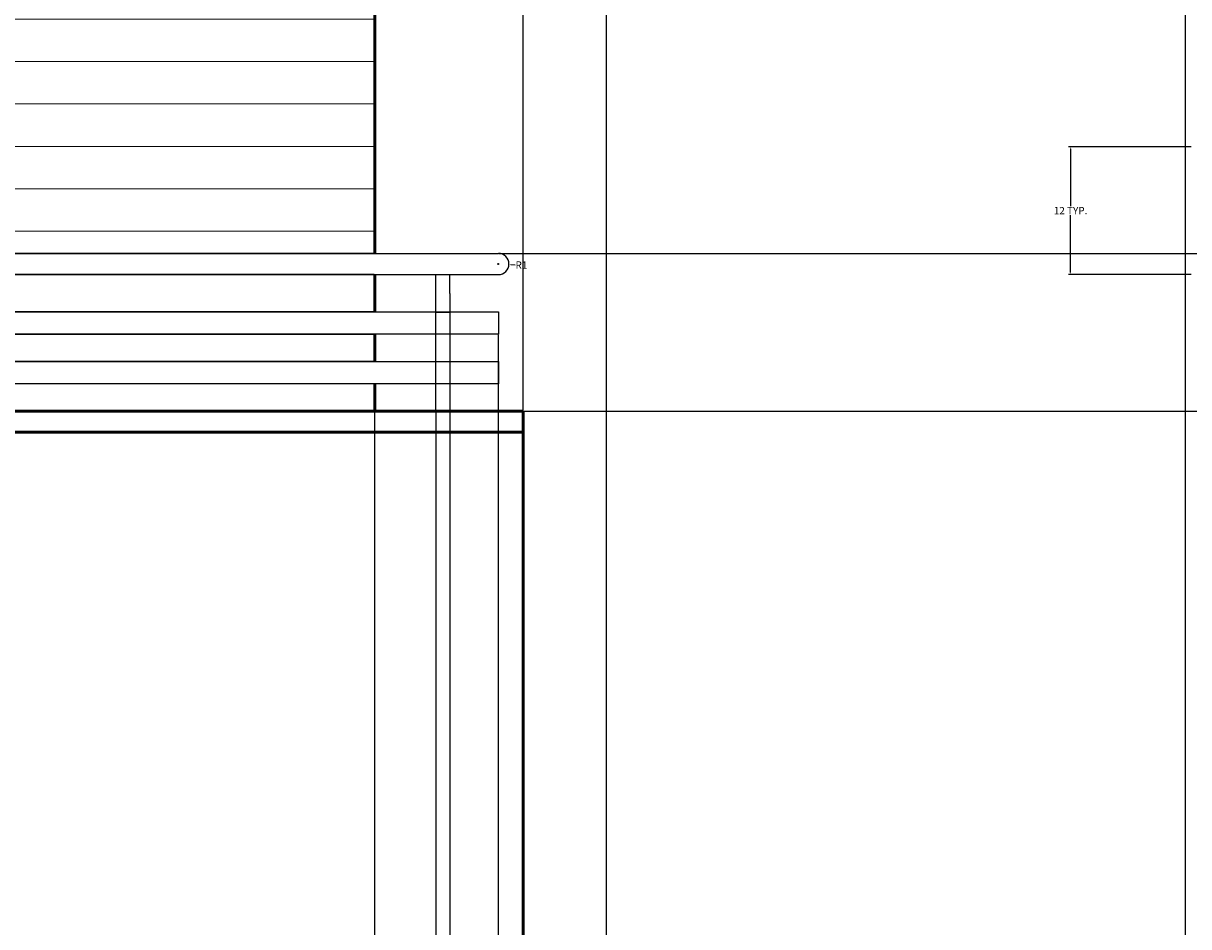
# Model space of a CAD drawing. Units: inches. Extents: x -139 to 346, y 72 to 413.
# Tile 9 of 18: x 66 to 175, y 242 to 328. Entities that reach past the tile are written whole.
import ezdxf

# ---------------------------------------------------------------- set-up
doc = ezdxf.new("R2010")
doc.units = ezdxf.units.IN
doc.header["$MEASUREMENT"] = 0
for name, color, linetype, lineweight in [('A-ANNO-DIMS', 2, 'Continuous', 18), ('A-ELEV-RAIL', 6, 'Continuous', 25), ('A-WALL', 7, 'Continuous', 50), ('A-WALL-PATT', 8, 'Continuous', 13)]:
    doc.layers.add(name, color=color, linetype=linetype, lineweight=lineweight)
doc.styles.get("Standard").update_dxf_attribs({"font": 'arial.ttf'})
doc.dimstyles.get("Standard").update_dxf_attribs({"dimtxt": 0.6875, "dimasz": 0.18, "dimexe": 0.18, "dimexo": 0.0625, "dimgap": 0.09, "dimtad": 0, "dimtih": 1, "dimtoh": 1, "dimdec": 4, "dimzin": 0, "dimdsep": 46, "dimlunit": 4, "dimtxsty": 'Standard', "dimcen": 0.09, "dimadec": 0, "dimazin": 0, "dimtfac": 1, "dimtdec": 4, "dimtofl": 0, "dimtmove": 0, "dimatfit": 3, "dimfxl": 1, "dimtolj": 1, "dimtzin": 0, "dimarcsym": 0})

# ---------------------------------------------------------------- blocks, each defined once
blk = doc.blocks.new('*D4')
at = {"layer": 'A-ANNO-DIMS', "color": 0, "lineweight": -2, "transparency": 16777216}
for p, q in [((175.61, 315.96), (164.06, 315.96)), ((164.24, 315.78), (164.24, 310.38)), ((164.24, 304.12), (164.24, 309.51)), ((175.61, 303.94), (164.06, 303.94))]:
    blk.add_line(p, q, dxfattribs=at)
at = {"layer": 'A-ANNO-DIMS', "color": 0, "transparency": 16777216}
for points in [[(164.21, 315.78), (164.27, 315.78), (164.24, 315.96)], [(164.21, 304.12), (164.27, 304.12), (164.24, 303.94)]]:
    blk.add_solid(points, dxfattribs=at)
at = {"layer": 'Defpoints', "color": 0, "transparency": 16777216}
for p in [(164.24, 315.96), (175.67, 315.96), (175.67, 303.94)]:
    blk.add_point(p, dxfattribs=at)
at = {"layer": 'A-ANNO-DIMS', "color": 0, "transparency": 16777216, "insert": (164.24, 309.95), "char_height": 0.6875, "attachment_point": 5}
blk.add_mtext('\\A1;12 TYP.', dxfattribs=at)
blk = doc.blocks.new('*D26')
at = {"layer": 'A-ANNO-DIMS', "color": 0, "lineweight": -2, "transparency": 16777216}
for p, q in [((98.67, 360.61), (98.67, 412.45)), ((98.85, 412.27), (104.18, 412.27)), ((112.47, 412.27), (107.15, 412.27)), ((112.65, 291.12), (112.65, 412.45))]:
    blk.add_line(p, q, dxfattribs=at)
at = {"layer": 'A-ANNO-DIMS', "color": 0, "transparency": 16777216}
for points in [[(98.85, 412.3), (98.85, 412.24), (98.67, 412.27)], [(112.47, 412.3), (112.47, 412.24), (112.65, 412.27)]]:
    blk.add_solid(points, dxfattribs=at)
at = {"layer": 'Defpoints', "color": 0, "transparency": 16777216}
for p in [(112.65, 412.27), (98.67, 360.54), (112.65, 291.06)]:
    blk.add_point(p, dxfattribs=at)
at = {"layer": 'A-ANNO-DIMS', "color": 0, "transparency": 16777216, "insert": (105.66, 412.27), "char_height": 0.688, "attachment_point": 5}
blk.add_mtext('\\A1;13.978', dxfattribs=at)
blk = doc.blocks.new('*D27')
at = {"layer": 'A-ANNO-DIMS', "color": 0, "lineweight": -2, "transparency": 16777216}
for p, q in [((112.65, 291.12), (112.65, 412.45)), ((112.83, 412.27), (142.91, 412.27)), ((175.49, 412.27), (145.41, 412.27)), ((175.67, 340.12), (175.67, 412.45))]:
    blk.add_line(p, q, dxfattribs=at)
at = {"layer": 'A-ANNO-DIMS', "color": 0, "transparency": 16777216}
for points in [[(112.83, 412.3), (112.83, 412.24), (112.65, 412.27)], [(175.49, 412.3), (175.49, 412.24), (175.67, 412.27)]]:
    blk.add_solid(points, dxfattribs=at)
at = {"layer": 'Defpoints', "color": 0, "transparency": 16777216}
for p in [(175.67, 412.27), (175.67, 340.05), (112.65, 291.06)]:
    blk.add_point(p, dxfattribs=at)
at = {"layer": 'A-ANNO-DIMS', "color": 0, "transparency": 16777216, "insert": (144.16, 412.27), "char_height": 0.688, "attachment_point": 5}
blk.add_mtext('\\A1;63.02', dxfattribs=at)
blk = doc.blocks.new('*D69')
at = {"layer": 'A-ANNO-DIMS', "color": 0, "lineweight": -2, "transparency": 16777216}
for p, q in [((120.51, 231.12), (120.51, 412.45)), ((120.69, 412.27), (146.54, 412.27)), ((174.89, 412.27), (149.04, 412.27)), ((175.07, 231.12), (175.07, 412.45))]:
    blk.add_line(p, q, dxfattribs=at)
at = {"layer": 'A-ANNO-DIMS', "color": 0, "transparency": 16777216}
for points in [[(120.69, 412.3), (120.69, 412.24), (120.51, 412.27)], [(174.89, 412.3), (174.89, 412.24), (175.07, 412.27)]]:
    blk.add_solid(points, dxfattribs=at)
at = {"layer": 'Defpoints', "color": 0, "transparency": 16777216}
for p in [(175.07, 412.27), (120.51, 231.06), (175.07, 231.06)]:
    blk.add_point(p, dxfattribs=at)
at = {"layer": 'A-ANNO-DIMS', "color": 0, "transparency": 16777216, "insert": (147.79, 412.27), "char_height": 0.688, "attachment_point": 5}
blk.add_mtext('\\A1;54.57', dxfattribs=at)
blk = doc.blocks.new('*D95')
at = {"layer": 'A-ANNO-DIMS', "color": 0, "lineweight": -2, "transparency": 16777216}
for p, q in [((98.61, 293.63), (-137.3, 293.63)), ((-137.12, 293.45), (-137.12, 292.78)), ((98.61, 291.06), (-137.3, 291.06)), ((-137.12, 291.24), (-137.12, 291.9))]:
    blk.add_line(p, q, dxfattribs=at)
at = {"layer": 'A-ANNO-DIMS', "color": 0, "transparency": 16777216}
for points in [[(-137.15, 293.45), (-137.09, 293.45), (-137.12, 293.63)], [(-137.15, 291.24), (-137.09, 291.24), (-137.12, 291.06)]]:
    blk.add_solid(points, dxfattribs=at)
at = {"layer": 'Defpoints', "color": 0, "transparency": 16777216}
for p in [(-137.12, 293.63), (98.67, 293.63), (98.67, 291.06)]:
    blk.add_point(p, dxfattribs=at)
at = {"layer": 'A-ANNO-DIMS', "color": 0, "transparency": 16777216, "insert": (-137.12, 292.34), "char_height": 0.688, "attachment_point": 5}
blk.add_mtext('\\A1;2.566', dxfattribs=at)
blk = doc.blocks.new('*D96')
at = {"layer": 'A-ANNO-DIMS', "color": 0, "lineweight": -2, "transparency": 16777216}
for p, q in [((98.61, 295.74), (-137.3, 295.74)), ((-137.12, 295.56), (-137.12, 295.12)), ((98.61, 293.63), (-137.3, 293.63)), ((-137.12, 293.81), (-137.12, 294.25))]:
    blk.add_line(p, q, dxfattribs=at)
at = {"layer": 'A-ANNO-DIMS', "color": 0, "transparency": 16777216}
for points in [[(-137.15, 295.56), (-137.09, 295.56), (-137.12, 295.74)], [(-137.15, 293.81), (-137.09, 293.81), (-137.12, 293.63)]]:
    blk.add_solid(points, dxfattribs=at)
at = {"layer": 'Defpoints', "color": 0, "transparency": 16777216}
for p in [(-137.12, 295.74), (98.67, 295.74), (98.67, 293.63)]:
    blk.add_point(p, dxfattribs=at)
at = {"layer": 'A-ANNO-DIMS', "color": 0, "transparency": 16777216, "insert": (-137.12, 294.68), "char_height": 0.688, "attachment_point": 5}
blk.add_mtext('\\A1;2.11', dxfattribs=at)
blk = doc.blocks.new('*D97')
at = {"layer": 'A-ANNO-DIMS', "color": 0, "lineweight": -2, "transparency": 16777216}
for p, q in [((98.61, 298.29), (-137.3, 298.29)), ((-137.12, 298.11), (-137.12, 297.46)), ((-137.12, 295.92), (-137.12, 296.57)), ((98.61, 295.74), (-137.3, 295.74))]:
    blk.add_line(p, q, dxfattribs=at)
at = {"layer": 'A-ANNO-DIMS', "color": 0, "transparency": 16777216}
for points in [[(-137.15, 298.11), (-137.09, 298.11), (-137.12, 298.29)], [(-137.15, 295.92), (-137.09, 295.92), (-137.12, 295.74)]]:
    blk.add_solid(points, dxfattribs=at)
at = {"layer": 'Defpoints', "color": 0, "transparency": 16777216}
for p in [(-137.12, 298.29), (98.67, 298.29), (98.67, 295.74)]:
    blk.add_point(p, dxfattribs=at)
at = {"layer": 'A-ANNO-DIMS', "color": 0, "transparency": 16777216, "insert": (-137.12, 297.02), "char_height": 0.688, "attachment_point": 5}
blk.add_mtext('\\A1;2.555', dxfattribs=at)
blk = doc.blocks.new('*D98')
at = {"layer": 'A-ANNO-DIMS', "color": 0, "lineweight": -2, "transparency": 16777216}
for p, q in [((98.61, 300.4), (-137.3, 300.4)), ((-137.12, 300.22), (-137.12, 299.78)), ((-137.12, 298.47), (-137.12, 298.91)), ((98.61, 298.29), (-137.3, 298.29))]:
    blk.add_line(p, q, dxfattribs=at)
at = {"layer": 'A-ANNO-DIMS', "color": 0, "transparency": 16777216}
for points in [[(-137.15, 300.22), (-137.09, 300.22), (-137.12, 300.4)], [(-137.15, 298.47), (-137.09, 298.47), (-137.12, 298.29)]]:
    blk.add_solid(points, dxfattribs=at)
at = {"layer": 'Defpoints', "color": 0, "transparency": 16777216}
for p in [(-137.12, 300.4), (98.67, 300.4), (98.67, 298.29)]:
    blk.add_point(p, dxfattribs=at)
at = {"layer": 'A-ANNO-DIMS', "color": 0, "transparency": 16777216, "insert": (-137.12, 299.35), "char_height": 0.688, "attachment_point": 5}
blk.add_mtext('\\A1;2.11', dxfattribs=at)
blk = doc.blocks.new('*D99')
at = {"layer": 'A-ANNO-DIMS', "color": 0, "lineweight": -2, "transparency": 16777216}
for p, q in [((98.61, 303.92), (-137.3, 303.92)), ((-137.12, 303.74), (-137.12, 302.6)), ((-137.12, 300.58), (-137.12, 301.72)), ((98.61, 300.4), (-137.3, 300.4))]:
    blk.add_line(p, q, dxfattribs=at)
at = {"layer": 'A-ANNO-DIMS', "color": 0, "transparency": 16777216}
for points in [[(-137.15, 303.74), (-137.09, 303.74), (-137.12, 303.92)], [(-137.15, 300.58), (-137.09, 300.58), (-137.12, 300.4)]]:
    blk.add_solid(points, dxfattribs=at)
at = {"layer": 'Defpoints', "color": 0, "transparency": 16777216}
for p in [(-137.12, 303.92), (98.67, 303.92), (98.67, 300.4)]:
    blk.add_point(p, dxfattribs=at)
at = {"layer": 'A-ANNO-DIMS', "color": 0, "transparency": 16777216, "insert": (-137.12, 302.16), "char_height": 0.688, "attachment_point": 5}
blk.add_mtext('\\A1;3.516', dxfattribs=at)
blk = doc.blocks.new('*D100')
at = {"layer": 'A-ANNO-DIMS', "color": 0, "lineweight": -2, "transparency": 16777216}
for p, q in [((98.61, 305.92), (-137.3, 305.92)), ((-137.12, 305.74), (-137.12, 305.36)), ((-137.12, 304.1), (-137.12, 304.49)), ((98.61, 303.92), (-137.3, 303.92))]:
    blk.add_line(p, q, dxfattribs=at)
at = {"layer": 'A-ANNO-DIMS', "color": 0, "transparency": 16777216}
for points in [[(-137.15, 305.74), (-137.09, 305.74), (-137.12, 305.92)], [(-137.15, 304.1), (-137.09, 304.1), (-137.12, 303.92)]]:
    blk.add_solid(points, dxfattribs=at)
at = {"layer": 'Defpoints', "color": 0, "transparency": 16777216}
for p in [(-137.12, 305.92), (98.67, 305.92), (98.67, 303.92)]:
    blk.add_point(p, dxfattribs=at)
at = {"layer": 'A-ANNO-DIMS', "color": 0, "transparency": 16777216, "insert": (-137.12, 304.92), "char_height": 0.688, "attachment_point": 5}
blk.add_mtext('\\A1;2', dxfattribs=at)
blk = doc.blocks.new('*D101')
at = {"layer": 'A-ANNO-DIMS', "color": 0, "lineweight": -2, "transparency": 16777216}
for p, q in [((110.39, 305.92), (344.39, 305.92)), ((344.21, 305.74), (344.21, 298.93)), ((344.21, 291.24), (344.21, 298.05)), ((112.71, 291.06), (344.39, 291.06))]:
    blk.add_line(p, q, dxfattribs=at)
at = {"layer": 'A-ANNO-DIMS', "color": 0, "transparency": 16777216}
for points in [[(344.18, 305.74), (344.24, 305.74), (344.21, 305.92)], [(344.18, 291.24), (344.24, 291.24), (344.21, 291.06)]]:
    blk.add_solid(points, dxfattribs=at)
at = {"layer": 'Defpoints', "color": 0, "transparency": 16777216}
for p in [(110.32, 305.92), (344.21, 305.92), (112.65, 291.06)]:
    blk.add_point(p, dxfattribs=at)
at = {"layer": 'A-ANNO-DIMS', "color": 0, "transparency": 16777216, "insert": (344.21, 298.49), "char_height": 0.688, "attachment_point": 5}
blk.add_mtext('\\A1;14.86', dxfattribs=at)
blk = doc.blocks.new('*D102')
at = {"layer": 'A-ANNO-DIMS', "color": 0, "lineweight": -2, "transparency": 16777216}
for p, q in [((98.67, 291), (98.67, 72.49)), ((104.42, 291), (104.42, 72.49)), ((98.85, 72.67), (100.3, 72.67)), ((104.24, 72.67), (102.79, 72.67))]:
    blk.add_line(p, q, dxfattribs=at)
at = {"layer": 'A-ANNO-DIMS', "color": 0, "transparency": 16777216}
for points in [[(98.85, 72.7), (98.85, 72.64), (98.67, 72.67)], [(104.24, 72.7), (104.24, 72.64), (104.42, 72.67)]]:
    blk.add_solid(points, dxfattribs=at)
at = {"layer": 'Defpoints', "color": 0, "transparency": 16777216}
for p in [(98.67, 291.06), (104.42, 291.06), (104.42, 72.67)]:
    blk.add_point(p, dxfattribs=at)
at = {"layer": 'A-ANNO-DIMS', "color": 0, "transparency": 16777216, "insert": (101.55, 72.67), "char_height": 0.688, "attachment_point": 5}
blk.add_mtext('\\A1;5.752', dxfattribs=at)
blk = doc.blocks.new('*D103')
at = {"layer": 'A-ANNO-DIMS', "color": 0, "lineweight": -2, "transparency": 16777216}
for p, q in [((104.42, 291), (104.42, 72.49)), ((105.74, 291), (105.74, 72.49)), ((104.6, 72.67), (105.56, 72.67)), ((105.74, 72.67), (105.92, 72.67))]:
    blk.add_line(p, q, dxfattribs=at)
at = {"layer": 'A-ANNO-DIMS', "color": 0, "transparency": 16777216}
for points in [[(104.6, 72.7), (104.6, 72.64), (104.42, 72.67)], [(105.56, 72.7), (105.56, 72.64), (105.74, 72.67)]]:
    blk.add_solid(points, dxfattribs=at)
at = {"layer": 'Defpoints', "color": 0, "transparency": 16777216}
for p in [(104.42, 291.06), (105.74, 291.06), (105.74, 72.67)]:
    blk.add_point(p, dxfattribs=at)
at = {"layer": 'A-ANNO-DIMS', "color": 0, "transparency": 16777216, "insert": (106.87, 72.67), "char_height": 0.688, "attachment_point": 5}
blk.add_mtext('\\A1;1.32', dxfattribs=at)
blk = doc.blocks.new('*D104')
at = {"layer": 'A-ANNO-DIMS', "color": 0, "lineweight": -2, "transparency": 16777216}
for p, q in [((110.32, 298.23), (110.32, 72.49)), ((105.74, 291), (105.74, 72.49)), ((105.92, 72.67), (106.77, 72.67)), ((110.14, 72.67), (109.29, 72.67))]:
    blk.add_line(p, q, dxfattribs=at)
at = {"layer": 'A-ANNO-DIMS', "color": 0, "transparency": 16777216}
for points in [[(105.92, 72.7), (105.92, 72.64), (105.74, 72.67)], [(110.14, 72.7), (110.14, 72.64), (110.32, 72.67)]]:
    blk.add_solid(points, dxfattribs=at)
at = {"layer": 'Defpoints', "color": 0, "transparency": 16777216}
for p in [(110.32, 298.29), (105.74, 291.06), (110.32, 72.67)]:
    blk.add_point(p, dxfattribs=at)
at = {"layer": 'A-ANNO-DIMS', "color": 0, "transparency": 16777216, "insert": (108.03, 72.67), "char_height": 0.688, "attachment_point": 5}
blk.add_mtext('\\A1;4.582', dxfattribs=at)
blk = doc.blocks.new('*D105')
at = {"layer": 'A-ANNO-DIMS', "color": 0, "lineweight": -2, "transparency": 16777216}
for p, q in [((110.32, 298.23), (110.32, 72.49)), ((112.65, 289), (112.65, 72.49)), ((110.5, 72.67), (112.47, 72.67)), ((112.65, 72.67), (112.83, 72.67))]:
    blk.add_line(p, q, dxfattribs=at)
at = {"layer": 'A-ANNO-DIMS', "color": 0, "transparency": 16777216}
for points in [[(110.5, 72.7), (110.5, 72.64), (110.32, 72.67)], [(112.47, 72.7), (112.47, 72.64), (112.65, 72.67)]]:
    blk.add_solid(points, dxfattribs=at)
at = {"layer": 'Defpoints', "color": 0, "transparency": 16777216}
for p in [(110.32, 298.29), (112.65, 289.06), (112.65, 72.67)]:
    blk.add_point(p, dxfattribs=at)
at = {"layer": 'A-ANNO-DIMS', "color": 0, "transparency": 16777216, "insert": (114.09, 72.67), "char_height": 0.688, "attachment_point": 5}
blk.add_mtext('\\A1;2.326', dxfattribs=at)
blk = doc.blocks.new('*D106')
at = {"layer": 'A-ANNO-DIMS', "color": 0, "lineweight": -2, "transparency": 16777216}
for p, q in [((110.23, 304.92), (110.41, 304.92)), ((110.32, 304.83), (110.32, 305.01)), ((111.92, 304.82), (111.5, 304.84))]:
    blk.add_line(p, q, dxfattribs=at)
at = {"layer": 'A-ANNO-DIMS', "color": 0, "transparency": 16777216}
blk.add_solid([(111.5, 304.87), (111.5, 304.81), (111.32, 304.86)], dxfattribs=at)
at = {"layer": 'Defpoints', "color": 0, "transparency": 16777216}
for p in [(110.32, 304.92), (111.32, 304.86)]:
    blk.add_point(p, dxfattribs=at)
at = {"layer": 'A-ANNO-DIMS', "color": 0, "transparency": 16777216, "insert": (112.5, 304.82), "char_height": 0.688, "attachment_point": 5}
blk.add_mtext('\\A1;R1', dxfattribs=at)

msp = doc.modelspace()

# ---------------------------------------------------------------- hatches: boundary and pattern name
at = {"layer": 'A-WALL-PATT'}
h = msp.add_hatch(dxfattribs=at)
h.set_pattern_fill('ANSI31', color=256, scale=32, angle=135)
h.paths.add_polyline_path([(98.6724, 360.5443), (-34.7346, 360.5443), (-34.7346, 353.0644), (-34.7346, 305.9205), (5.6729, 305.9205), (5.6729, 338.3217), (62.4258, 338.3217), (62.4258, 305.9205), (98.6724, 305.9205)])
h.paths.add_polyline_path([(212.769, 231.0607), (175.072, 231.0607), (175.072, 218.0635), (171.0337, 218.0635), (171.0337, 115.6761), (125.2464, 115.6761), (125.2464, 218.0635), (123.4318, 218.0635), (120.5054, 218.0635), (120.5054, 231.0607), (112.6506, 231.0607), (112.6506, 112.6042), (212.769, 112.6042)])

# ---------------------------------------------------------------- linework, layer by layer
at = {"layer": 'A-ELEV-RAIL'}
for p, q in [((-44.6423, 305.9205), (110.3243, 305.9205)), ((-44.6423, 303.9205), (110.3243, 303.9205)), ((104.4244, 302.1482), (104.4244, 303.9205)), ((105.7421, 302.1482), (105.7421, 303.9205)), ((104.4244, 300.3938), (104.4244, 302.1482)), ((105.7421, 302.1482), (105.7421, 300.3938)), ((104.4244, 291.0604), (104.4244, 300.3938)), ((104.4244, 300.3938), (105.7421, 300.3938)), ((105.7421, 300.3938), (105.7421, 291.0604))]:
    msp.add_line(p, q, dxfattribs=at)
for points in [[(-44.2923, 300.4047), (110.3243, 300.4047), (110.3243, 298.293), (-44.2923, 298.293)], [(-44.2923, 295.7379), (110.3243, 295.7379), (110.3243, 293.6263), (-44.2923, 293.6263)]]:
    msp.add_lwpolyline(points, close=True, dxfattribs=at)
msp.add_arc((110.3243, 304.9205), 1, 270, 90, dxfattribs=at)
at = {"layer": 'A-WALL'}
for p, q in [((98.6724, 305.9205), (98.6724, 382.9748)), ((98.6724, 300.4047), (98.6724, 303.9205)), ((98.6724, 295.7379), (98.6724, 298.293)), ((98.6724, 291.0604), (98.6724, 293.6263)), ((112.6506, 291.0604), (-47.2734, 291.0604)), ((112.6506, 274.9748), (112.6506, 291.0604)), ((112.6506, 289.0604), (-47.2734, 289.0604)), ((112.6506, 238.9748), (112.6506, 274.9748))]:
    msp.add_line(p, q, dxfattribs=at)

# ---------------------------------------------------------------- dimensions: what is measured, and where the dimension line sits
at = {"layer": 'A-ANNO-DIMS'}
for base, p1, p2, override, picture, middle in [((112.6506, 412.2748), (98.6724, 360.5443), (112.6506, 291.0604), {"dimdec": 3, "dimlfac": 1, "dimrnd": 0, "dimzin": 0, "dimdsep": 46, "dimlunit": 2}, '*D26', (105.6615, 412.2748)), ((175.6676, 412.2748), (112.6506, 291.0604), (175.6676, 340.0548), {"dimdec": 2, "dimlfac": 1, "dimrnd": 0, "dimzin": 0, "dimdsep": 46, "dimlunit": 2}, '*D27', (144.1591, 412.2748)), ((175.072, 412.2748), (120.5054, 231.0607), (175.072, 231.0607), {"dimdec": 2, "dimlfac": 1, "dimrnd": 0, "dimzin": 0, "dimdsep": 46, "dimlunit": 2}, '*D69', (147.7887, 412.2748)), ((110.3243, 72.6748), (105.7421, 291.0604), (110.3243, 298.293), {"dimdec": 3, "dimlfac": 1, "dimrnd": 0, "dimzin": 0, "dimdsep": 46, "dimlunit": 2}, '*D104', (108.0332, 72.6748)), ((112.6506, 72.6748), (110.3243, 298.293), (112.6506, 289.0604), {"dimdec": 3, "dimlfac": 1, "dimrnd": 0, "dimzin": 0, "dimdsep": 46, "dimlunit": 2}, '*D105', (114.0862, 72.6748)), ((104.4244, 72.6748), (98.6724, 291.0604), (104.4244, 291.0604), {"dimdec": 3, "dimlfac": 1, "dimrnd": 0, "dimzin": 0, "dimdsep": 46, "dimlunit": 2}, '*D102', (101.5484, 72.6748)), ((105.7421, 72.6748), (104.4244, 291.0604), (105.7421, 291.0604), {"dimdec": 2, "dimlfac": 1, "dimrnd": 0, "dimzin": 0, "dimdsep": 46, "dimlunit": 2}, '*D103', (106.8691, 72.6748))]:
    dim = msp.add_linear_dim(base=base, p1=p1, p2=p2, dimstyle='Standard', override=override, dxfattribs=at)
    dim.commit()
    dim.dimension.update_dxf_attribs({"geometry": picture, "text_midpoint": middle})
dim = msp.add_linear_dim(base=(164.2442, 315.9552), p1=(175.6676, 303.9402), p2=(175.6676, 315.9552), angle=90, text='<> TYP.', dimstyle='Standard', override={"dimdec": 0, "dimlfac": 1, "dimrnd": 0, "dimzin": 0, "dimdsep": 46, "dimlunit": 2}, dxfattribs=at)
dim.commit()
dim.dimension.update_dxf_attribs({"geometry": '*D4', "text_midpoint": (164.2442, 309.9477)})
for base, p1, p2, override, picture, middle in [((-137.1237, 305.9205), (98.6724, 303.9205), (98.6724, 305.9205), {"dimdec": 0, "dimlfac": 1, "dimrnd": 0, "dimzin": 0, "dimdsep": 46, "dimlunit": 2}, '*D100', (-137.1237, 304.9205)), ((344.2055, 305.9205), (112.6506, 291.0604), (110.3243, 305.9205), {"dimdec": 2, "dimlfac": 1, "dimrnd": 0, "dimzin": 0, "dimdsep": 46, "dimlunit": 2}, '*D101', (344.2055, 298.4905)), ((-137.1237, 303.9205), (98.6724, 300.4047), (98.6724, 303.9205), {"dimdec": 3, "dimlfac": 1, "dimrnd": 0, "dimzin": 0, "dimdsep": 46, "dimlunit": 2}, '*D99', (-137.1237, 302.1626)), ((-137.1237, 300.4047), (98.6724, 298.293), (98.6724, 300.4047), {"dimdec": 2, "dimlfac": 1, "dimrnd": 0, "dimzin": 0, "dimdsep": 46, "dimlunit": 2}, '*D98', (-137.1237, 299.3488)), ((-137.1237, 298.293), (98.6724, 295.7379), (98.6724, 298.293), {"dimdec": 3, "dimlfac": 1, "dimrnd": 0, "dimzin": 0, "dimdsep": 46, "dimlunit": 2}, '*D97', (-137.1237, 297.0155)), ((-137.1237, 295.7379), (98.6724, 293.6263), (98.6724, 295.7379), {"dimdec": 2, "dimlfac": 1, "dimrnd": 0, "dimzin": 0, "dimdsep": 46, "dimlunit": 2}, '*D96', (-137.1237, 294.6821)), ((-137.1237, 293.6263), (98.6724, 291.0604), (98.6724, 293.6263), {"dimdec": 3, "dimlfac": 1, "dimrnd": 0, "dimzin": 0, "dimdsep": 46, "dimlunit": 2}, '*D95', (-137.1237, 292.3433))]:
    dim = msp.add_linear_dim(base=base, p1=p1, p2=p2, angle=90, dimstyle='Standard', override=override, dxfattribs=at)
    dim.commit()
    dim.dimension.update_dxf_attribs({"geometry": picture, "text_midpoint": middle})
dim = msp.add_radius_dim(center=(110.3243, 304.9205), mpoint=(111.3222, 304.8551), dimstyle='Standard', override={"dimdec": 0, "dimlfac": 1, "dimrnd": 0, "dimzin": 0, "dimdsep": 46, "dimlunit": 2}, dxfattribs=at)
dim.commit()
dim.dimension.update_dxf_attribs({"geometry": '*D106', "text_midpoint": (111.9209, 304.8159), "dimtype": 164})

doc.saveas('drawing.dxf')
